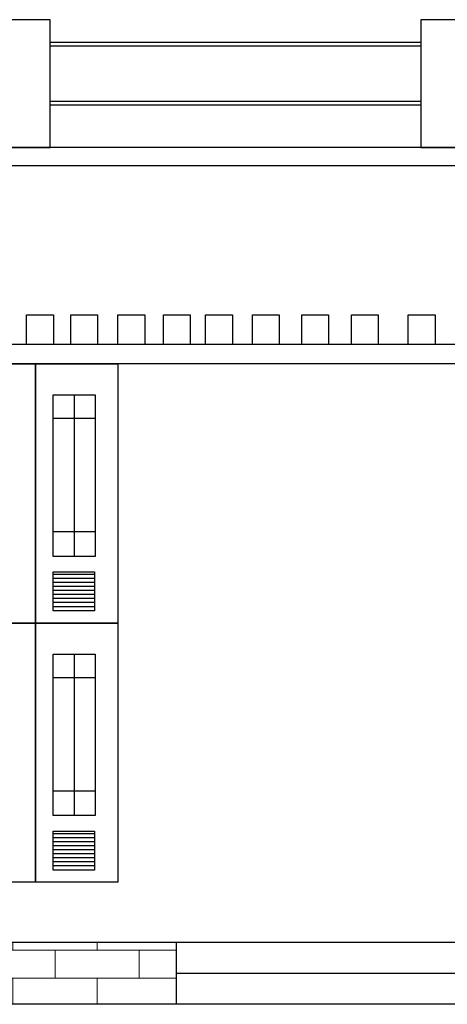
# Model space of a CAD drawing. Units: metres. Extents: x 10365 to 12529, y 3661 to 6248.
# Tile 5 of 9: x 10987 to 11333, y 4875 to 5673. Entities that reach past the tile are written whole.
import ezdxf

# ---------------------------------------------------------------- set-up
doc = ezdxf.new("R2010")
doc.units = ezdxf.units.M
doc.header["$MEASUREMENT"] = 0
doc.layers.add('A-ELEV', color=7, linetype='Continuous', lineweight=25)
doc.layers.add('A-ELEV-PATT', color=8, linetype='Continuous', lineweight=13)

# ---------------------------------------------------------------- blocks, each defined once
blk = doc.blocks.new('ELEV-DENTIL')
for p, q in [((0, 0), (0, 23.79)), ((0, 23.79), (21.67, 23.79)), ((21.67, 23.79), (21.67, 0))]:
    blk.add_line(p, q)

msp = doc.modelspace()

# ---------------------------------------------------------------- hatches: boundary and pattern name
at = {"layer": 'A-ELEV-PATT'}
h = msp.add_hatch(dxfattribs=at)
h.set_pattern_fill('AR-BRSTD', color=256, scale=8.5)
h.paths.add_polyline_path([(11113.98, 4925.82), (10590.74, 4925.82), (10573.67, 4925.82), (10573.67, 4875.44), (11113.98, 4875.44)])

# ---------------------------------------------------------------- linework, layer by layer
at = {"layer": 'A-ELEV'}
for p, q in [((11012.02, 5654.29), (11312.04, 5654.29)), ((11012.02, 5651.29), (11312.04, 5651.29)), ((11012.02, 5606.51), (11312.04, 5606.51)), ((11012.02, 5603.51), (11312.04, 5603.51)), ((11343.22, 5569.17), (10563.57, 5569.17)), ((10590.74, 5409.77), (11343.22, 5409.77)), ((11343.22, 5394.05), (10590.74, 5394.05)), ((11031.52, 5368.73), (11031.52, 5238.09)), ((11014.54, 5349.84), (11048.49, 5349.84)), ((11014.54, 5258.3), (11048.49, 5258.3)), ((11014.54, 5223.7), (11047.98, 5223.7)), ((11014.54, 5220.44), (11047.98, 5220.44)), ((11014.54, 5217.18), (11047.98, 5217.18)), ((11014.54, 5213.92), (11047.98, 5213.92)), ((11014.54, 5210.66), (11047.98, 5210.66)), ((11014.54, 5207.4), (11047.98, 5207.4)), ((11014.54, 5204.13), (11047.98, 5204.13)), ((11014.54, 5204.13), (11047.98, 5204.13)), ((11014.54, 5200.87), (11047.98, 5200.87)), ((11014.54, 5197.61), (11047.98, 5197.61)), ((11031.52, 5158.81), (11031.52, 5028.16)), ((11014.54, 5139.92), (11048.49, 5139.92)), ((11014.54, 5048.38), (11048.49, 5048.38)), ((11014.54, 5013.78), (11047.98, 5013.78)), ((11014.54, 5010.52), (11047.98, 5010.52)), ((11014.54, 5007.26), (11047.98, 5007.26)), ((11014.54, 5003.99), (11047.98, 5003.99)), ((11014.54, 5000.73), (11047.98, 5000.73)), ((11014.54, 4997.47), (11047.98, 4997.47)), ((11014.54, 4994.21), (11047.98, 4994.21)), ((11014.54, 4994.21), (11047.98, 4994.21)), ((11014.54, 4990.95), (11047.98, 4990.95)), ((11014.54, 4987.69), (11047.98, 4987.69)), ((11113.98, 4925.82), (11113.98, 4875.44)), ((11113.98, 4900.63), (11343.22, 4900.63)), ((11343.22, 4875.44), (10573.67, 4875.44))]:
    msp.add_line(p, q, dxfattribs=at)
for points in [[(10978.4, 5569.17), (10978.4, 5569.17), (11012.02, 5569.17), (11012.02, 5569.17), (11012.02, 5672.53), (11012.02, 5672.53), (10978.4, 5672.53), (10978.4, 5672.53)], [(11312.04, 5569.17), (11312.04, 5569.17), (11345.66, 5569.17), (11345.66, 5569.17), (11345.66, 5672.53), (11345.66, 5672.53), (11312.04, 5672.53), (11312.04, 5672.53)], [(11343.22, 5554.17), (11343.22, 5554.17), (10590.74, 5554.17), (10590.74, 5554.17), (10590.74, 4925.82), (10590.74, 4925.82), (11343.22, 4925.82), (11343.22, 4925.82)], [(10933.68, 5394.05), (10933.68, 5394.05), (11000.28, 5394.05), (11000.28, 5394.05), (11000.28, 5184.13), (11000.28, 5184.13), (10933.68, 5184.13), (10933.68, 5184.13)], [(11000.28, 5394.05), (11000.28, 5394.05), (11066.88, 5394.05), (11066.88, 5394.05), (11066.88, 5184.13), (11066.88, 5184.13), (11000.28, 5184.13), (11000.28, 5184.13)], [(11014.54, 5368.73), (11014.54, 5368.73), (11048.49, 5368.73), (11048.49, 5368.73), (11048.49, 5238.09), (11048.49, 5238.09), (11014.54, 5238.09), (11014.54, 5238.09)], [(11014.54, 5225.53), (11014.54, 5225.53), (11047.98, 5225.53), (11047.98, 5225.53), (11047.98, 5194.04), (11047.98, 5194.04), (11014.54, 5194.04), (11014.54, 5194.04)], [(10933.68, 5184.13), (10933.68, 5184.13), (11000.28, 5184.13), (11000.28, 5184.13), (11000.28, 4974.2), (11000.28, 4974.2), (10933.68, 4974.2), (10933.68, 4974.2)], [(11000.28, 5184.13), (11000.28, 5184.13), (11066.88, 5184.13), (11066.88, 5184.13), (11066.88, 4974.2), (11066.88, 4974.2), (11000.28, 4974.2), (11000.28, 4974.2)], [(11014.54, 5158.81), (11014.54, 5158.81), (11048.49, 5158.81), (11048.49, 5158.81), (11048.49, 5028.16), (11048.49, 5028.16), (11014.54, 5028.16), (11014.54, 5028.16)], [(11014.54, 5015.6), (11014.54, 5015.6), (11047.98, 5015.6), (11047.98, 5015.6), (11047.98, 4984.11), (11047.98, 4984.11), (11014.54, 4984.11), (11014.54, 4984.11)]]:
    msp.add_lwpolyline(points, close=True, dxfattribs=at)

# ---------------------------------------------------------------- block references
for p in [(10993.03, 5409.77), (11028.85, 5409.77), (11066.93, 5409.77), (11103.65, 5409.77), (11137.81, 5409.77), (11175.69, 5409.77), (11215.55, 5409.77), (11255.84, 5409.77), (11301.79, 5409.77)]:
    msp.add_blockref('ELEV-DENTIL', p, dxfattribs=at)

doc.saveas('drawing.dxf')
